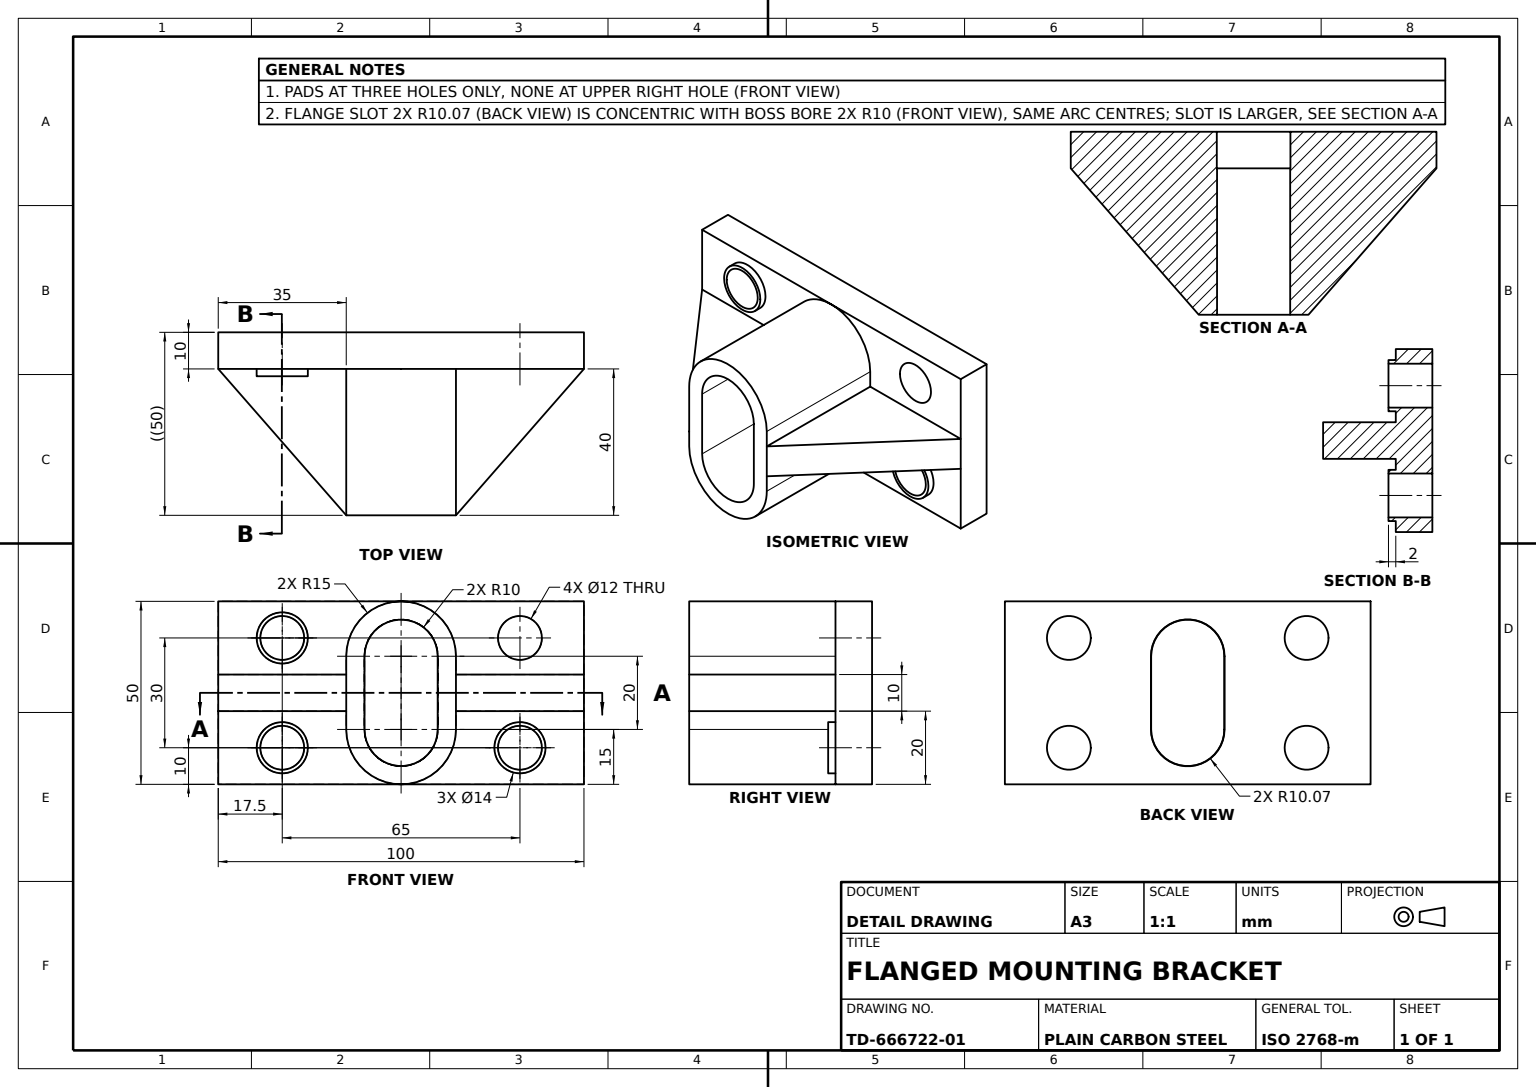
from build123d import *

# Parameters (mm, degrees)
BASE_PLATE_SKETCH_W         = 100
BASE_PLATE_SKETCH_H         = 50
BASE_PLATE_100X50X10_DEPTH  = 10
OVAL_BOSS_DEPTH             = 40
SUPPORT_RIB_1_REACH         = 116.564
SUPPORT_RIB_1_SKETCH_WALL_W = 284.279513812
SUPPORT_RIB_1_SKETCH_WALL_H = 10
SUPPORT_RIB_2_REACH         = 116.564
SUPPORT_RIB_2_SKETCH_WALL_W = 284.279513812
SUPPORT_RIB_2_SKETCH_WALL_H = 10
RAISED_PADS_SKETCH_R        = 7
RAISED_PADS_SKETCH_R_2      = 6
RAISED_PADS_2MM_DEPTH       = 2
MOUNTING_HOLE_1_SKETCH_R    = 6
MOUNTING_HOLE_1_DEPTH       = 119.74342087
MOUNTING_HOLE_2_SKETCH_R    = 6
MOUNTING_HOLE_2_DEPTH       = 119.74342087
MOUNTING_HOLE_3_SKETCH_R    = 6
MOUNTING_HOLE_3_DEPTH       = 119.084715353
MOUNTING_HOLE_4_SKETCH_R    = 6
MOUNTING_HOLE_4_DEPTH       = 119.74342087
BOSS_BORE_DEPTH             = 119.74342087


with BuildPart() as part:
    # Base Plate Sketch → Base Plate 100x50x10 (new body)
    with BuildSketch(Plane.XY):
        with Locations((50, 25)):
            Rectangle(BASE_PLATE_SKETCH_W, BASE_PLATE_SKETCH_H)
    extrude(amount=BASE_PLATE_100X50X10_DEPTH)

    # Oval Boss Sketch → Oval Boss (add)
    with BuildSketch(Plane.XY.offset(10)):
        with BuildLine():
            Line((35, 15), (35, 35))
            ThreePointArc((35, 35), (50, 50), (65, 35))
            Line((65, 35), (65, 15))
            ThreePointArc((65, 15), (50, 0), (35, 15))
        make_face()
        with BuildLine():
            Line((40, 15), (40, 35))
            ThreePointArc((40, 35), (50, 45), (60, 35))
            Line((60, 35), (60, 15))
            ThreePointArc((60, 15), (50, 5), (40, 15))
        make_face(mode=Mode.SUBTRACT)
    extrude(amount=OVAL_BOSS_DEPTH)

    # Support Rib 1 Sketch wall → Support Rib 1 (add, up to next)
    with BuildSketch(Plane(origin=(82.5, 25, 30), x_dir=(0.658504607869, 0, -0.752576694707), z_dir=(-0.752576694707, 0, -0.658504607869)), mode=Mode.PRIVATE) as support_rib_1_sk1:
        Rectangle(SUPPORT_RIB_1_SKETCH_WALL_W, SUPPORT_RIB_1_SKETCH_WALL_H)
    support_rib_1_tool1 = extrude(support_rib_1_sk1.sketch, amount=SUPPORT_RIB_1_REACH, mode=Mode.PRIVATE) - part.part
    add(support_rib_1_tool1.solids().sort_by_distance((82.5, 25, 30))[0])

    # Support Rib 2 Sketch wall → Support Rib 2 (add, up to next)
    with BuildSketch(Plane(origin=(17.5, 25, 30), x_dir=(-0.658504607869, 0, -0.752576694707), z_dir=(-0.752576694707, 0, 0.658504607869)), mode=Mode.PRIVATE) as support_rib_2_sk1:
        Rectangle(SUPPORT_RIB_2_SKETCH_WALL_W, SUPPORT_RIB_2_SKETCH_WALL_H)
    support_rib_2_tool1 = extrude(support_rib_2_sk1.sketch, amount=-SUPPORT_RIB_2_REACH, mode=Mode.PRIVATE) - part.part
    add(support_rib_2_tool1.solids().sort_by_distance((17.5, 25, 30))[0])

    # Raised Pads Sketch → Raised Pads 2mm (add)
    # profile 1 of 4: a face of its own
    with BuildSketch(Plane.XY.offset(10)):
        with Locations((17.5, 10)):
            Circle(RAISED_PADS_SKETCH_R)
        with Locations((17.5, 10)):
            Circle(RAISED_PADS_SKETCH_R_2, mode=Mode.SUBTRACT)
    # profile 2 of 4: a face of its own
    with BuildSketch(Plane.XY.offset(10)):
        with Locations((82.5, 10)):
            Circle(RAISED_PADS_SKETCH_R)
        with Locations((82.5, 10)):
            Circle(RAISED_PADS_SKETCH_R_2, mode=Mode.SUBTRACT)
    # profile 3 of 4: a face of its own
    with BuildSketch(Plane.XY.offset(10)):
        with Locations((17.5, 40)):
            Circle(RAISED_PADS_SKETCH_R)
        with Locations((17.5, 40)):
            Circle(RAISED_PADS_SKETCH_R_2, mode=Mode.SUBTRACT)
    # profile 4 of 4: a face of its own
    with BuildSketch(Plane.XY.offset(10)):
        with Locations((82.5, 40)):
            Circle(RAISED_PADS_SKETCH_R_2)
    extrude(amount=RAISED_PADS_2MM_DEPTH)

    # Mounting Hole 1 Sketch → Mounting Hole 1 (cut, through all)
    with BuildSketch(Plane.XY.offset(10)):
        with Locations((17.5, 40)):
            Circle(MOUNTING_HOLE_1_SKETCH_R)
    extrude(amount=-MOUNTING_HOLE_1_DEPTH, mode=Mode.SUBTRACT)

    # Mounting Hole 2 Sketch → Mounting Hole 2 (cut, through all)
    with BuildSketch(Plane.XY.offset(10)):
        with Locations((17.5, 10)):
            Circle(MOUNTING_HOLE_2_SKETCH_R)
    extrude(amount=-MOUNTING_HOLE_2_DEPTH, mode=Mode.SUBTRACT)

    # Mounting Hole 3 Sketch → Mounting Hole 3 (cut, through all)
    with BuildSketch(Plane.XY.offset(12)):
        with Locations((82.5, 40)):
            Circle(MOUNTING_HOLE_3_SKETCH_R)
    extrude(amount=-MOUNTING_HOLE_3_DEPTH, mode=Mode.SUBTRACT)

    # Mounting Hole 4 Sketch → Mounting Hole 4 (cut, through all)
    with BuildSketch(Plane.XY.offset(10)):
        with Locations((82.5, 10)):
            Circle(MOUNTING_HOLE_4_SKETCH_R)
    extrude(amount=-MOUNTING_HOLE_4_DEPTH, mode=Mode.SUBTRACT)

    # Boss Bore Sketch → Boss Bore (cut, through all)
    with BuildSketch(Plane.XY.offset(10)):
        with BuildLine():
            Line((39.934647115, 15), (39.934647115, 35))
            ThreePointArc((39.934647115, 35), (50, 45.065352885), (60.065352885, 35))
            Line((60.065352885, 35), (60.065352885, 15))
            ThreePointArc((60.065352885, 15), (50, 4.934647115), (39.934647115, 15))
        make_face()
    extrude(amount=-BOSS_BORE_DEPTH, mode=Mode.SUBTRACT)


solid = part.part
